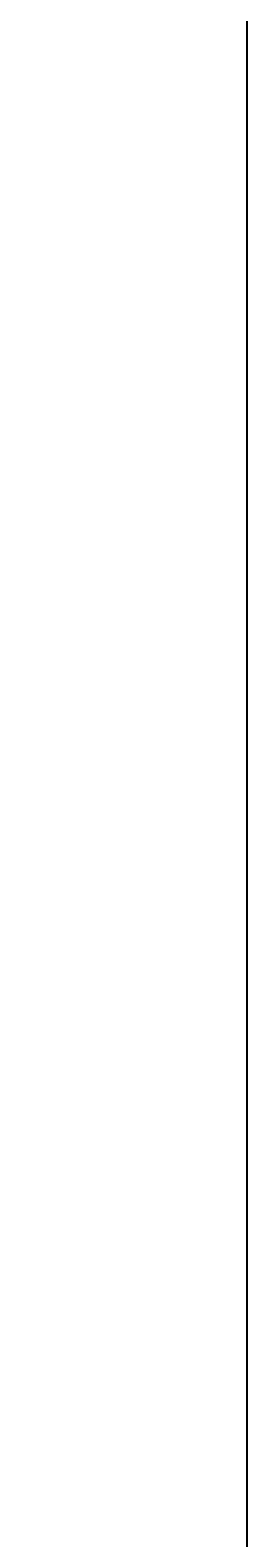
# Model space of a CAD drawing. Units: inches. Extents: x 2812 to 3051, y 1398 to 1659.
# Tile 11 of 65: x 2848 to 2852, y 1501 to 1528. Entities that reach past the tile are written whole.
import ezdxf

# ---------------------------------------------------------------- set-up
doc = ezdxf.new("R2010")
doc.units = ezdxf.units.IN
doc.layers.add('A-ANNO-DIMS', color=2, linetype='Continuous', lineweight=18)
doc.styles.get("Standard").update_dxf_attribs({"font": 'arial.ttf'})
doc.dimstyles.get("Standard").update_dxf_attribs({"dimtxt": 0.18, "dimasz": 0.18, "dimexe": 0.18, "dimexo": 0.0625, "dimgap": 0.09, "dimtad": 0, "dimtih": 1, "dimtoh": 1, "dimdec": 4, "dimzin": 0, "dimdsep": 46, "dimtxsty": 'Standard', "dimcen": 0.09, "dimadec": 0, "dimazin": 0, "dimtfac": 1, "dimtdec": 4, "dimtofl": 0, "dimtmove": 0, "dimatfit": 3, "dimfxl": 1, "dimtolj": 1, "dimtzin": 0, "dimarcsym": 0})

# ---------------------------------------------------------------- blocks, each defined once
blk = doc.blocks.new('*D28')
at = {"layer": 'A-ANNO-DIMS', "color": 0, "lineweight": -2, "transparency": 16777216}
for p, q in [((2851.646, 1598.667), (2851.646, 1397.505)), ((2844.385, 1559.757), (2844.385, 1397.505)), ((2844.565, 1397.685), (2847.64, 1397.685)), ((2851.466, 1397.685), (2848.391, 1397.685))]:
    blk.add_line(p, q, dxfattribs=at)
at = {"layer": 'A-ANNO-DIMS', "color": 0, "transparency": 16777216}
for points in [[(2844.565, 1397.715), (2844.565, 1397.655), (2844.385, 1397.685)], [(2851.466, 1397.715), (2851.466, 1397.655), (2851.646, 1397.685)]]:
    blk.add_solid(points, dxfattribs=at)
at = {"layer": 'Defpoints', "color": 0, "transparency": 16777216}
for p in [(2851.646, 1598.73), (2844.385, 1559.82), (2851.646, 1397.685)]:
    blk.add_point(p, dxfattribs=at)
at = {"layer": 'A-ANNO-DIMS', "color": 0, "transparency": 16777216, "insert": (2848.016, 1397.685), "char_height": 0.18, "attachment_point": 5}
blk.add_mtext('\\A1;7.261', dxfattribs=at)

msp = doc.modelspace()

# ---------------------------------------------------------------- dimensions: what is measured, and where the dimension line sits
at = {"layer": 'A-ANNO-DIMS'}
dim = msp.add_linear_dim(base=(2851.6462, 1397.6854), p1=(2844.3849, 1559.82), p2=(2851.6462, 1598.7296), dimstyle='Standard', override={"dimdec": 3, "dimlfac": 1, "dimrnd": 0, "dimzin": 0, "dimdsep": 46, "dimlunit": 2}, dxfattribs=at)
dim.commit()
dim.dimension.update_dxf_attribs({"geometry": '*D28', "text_midpoint": (2848.0156, 1397.6854)})

doc.saveas('drawing.dxf')
